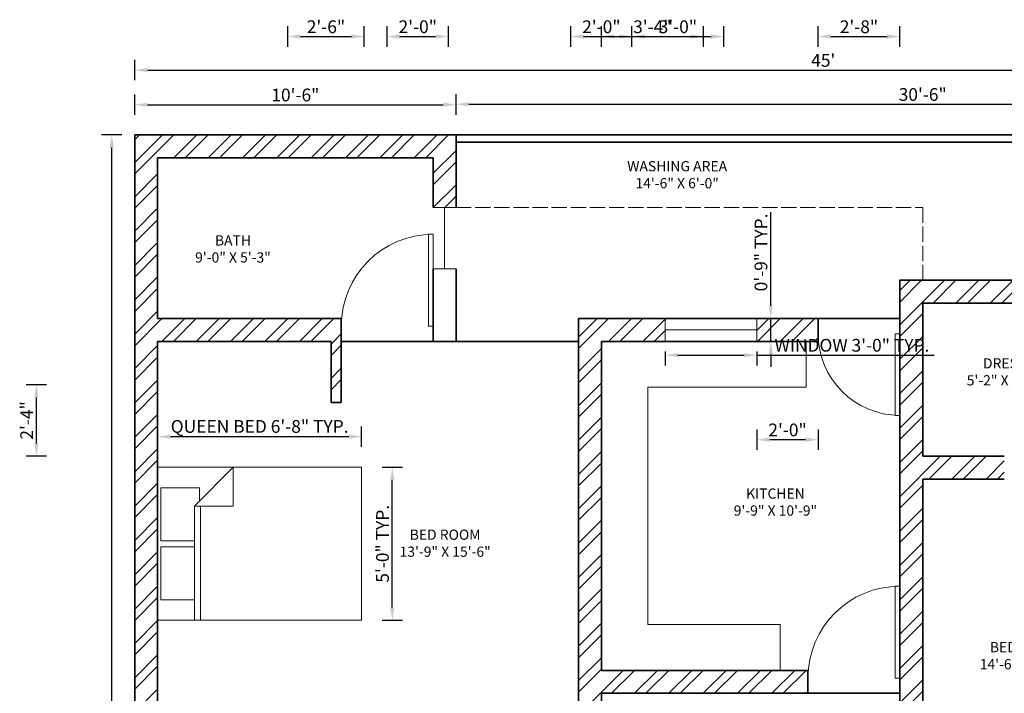
# Model space of a CAD drawing. Units: inches. Extents: x 468 to 1096, y 138 to 946.
# Tile 4 of 6: x 468 to 854, y 682 to 946. Entities that reach past the tile are written whole.
import ezdxf

# ---------------------------------------------------------------- set-up
doc = ezdxf.new("R2010")
doc.units = ezdxf.units.IN
doc.linetypes.add('ACAD_ISO02W100', pattern=[15, 12, -3])
for name, color, linetype, lineweight in [('A-ANNO-DIMS', 2, 'Continuous', 18), ('A-AREA-IDEN', 7, 'Continuous', 18), ('A-DOOR', 3, 'Continuous', 18), ('A-FLOR-CASE', 9, 'Continuous', 18), ('A-FURN', 8, 'Continuous', 18), ('A-GLAZ', 4, 'Continuous', 18), ('A-ROOF-OVHD', 7, 'ACAD_ISO02W100', 18), ('A-WALL', 7, 'Continuous', 35), ('A-WALL-PATT', 8, 'Continuous', 13), ('C-PROP', 7, 'Continuous', 35)]:
    doc.layers.add(name, color=color, linetype=linetype, lineweight=lineweight)
doc.styles.get("Standard").update_dxf_attribs({"font": 'arial.ttf'})
doc.dimstyles.new('ISO-25', dxfattribs={"dimtxt": 5, "dimasz": 5, "dimexe": 4, "dimexo": 4, "dimtad": 1, "dimdec": 1, "dimlunit": 3, "dimtxsty": 'Standard', "dimcen": 2.5, "dimadec": 0, "dimazin": 0, "dimtfac": 1, "dimtdec": 1, "dimtmove": 0, "dimatfit": 3, "dimfxl": 4, "dimfxlon": 1, "dimarcsym": 0})

# ---------------------------------------------------------------- blocks, each defined once
blk = doc.blocks.new('*U3')
for p, q in [((0, 0), (0, -6)), ((-36, 0), (-36, -6))]:
    blk.add_line(p, q)
blk.add_lwpolyline([(0, 0), (0, 36), (-1.75, 36), (-1.75, 0)], close=True)
blk.add_arc((0, 0), 36, 90, 180)
blk = doc.blocks.new('*U4')
for p, q in [((0, 0), (0, -6)), ((-32, 0), (-32, -6))]:
    blk.add_line(p, q)
blk.add_lwpolyline([(0, 0), (0, 32), (-1.75, 32), (-1.75, 0)], close=True)
blk.add_arc((0, 0), 32, 90, 180)
blk = doc.blocks.new('Bed - Queen')
for p, q in [((0, -80.00003), (0, 0)), ((0, 0), (59.99999, 0)), ((59.99999, 0), (59.99999, -80.00003)), ((7.99999, -1.2), (28.79998, -1.2)), ((7.99999, -14.4), (7.99999, -1.2)), ((28.79998, -1.2), (28.79998, -14.4)), ((31.19999, -1.2), (51.99999, -1.2)), ((31.19999, -14.4), (31.19999, -1.2)), ((51.99999, -1.2), (51.99999, -16.4)), ((0, -14.4), (44.8, -14.4)), ((59.99999, -29.6), (44.8, -14.4)), ((44.8, -14.4), (44.8, -29.6)), ((44.8, -16.8), (0, -16.8)), ((51.99999, -16.4), (46.79936, -16.4)), ((44.8, -29.6), (59.99999, -29.6)), ((59.99999, -80.00003), (0, -80.00003))]:
    blk.add_line(p, q)
blk = doc.blocks.new('*D15')
at = {"layer": 'A-ANNO-DIMS', "color": 0, "lineweight": -2, "transparency": 16777216}
for p, q in [((513.13, 908.95), (513.13, 916.95)), ((639.13, 908.95), (639.13, 916.95)), ((518.13, 912.95), (634.13, 912.95))]:
    blk.add_line(p, q, dxfattribs=at)
at = {"layer": 'A-ANNO-DIMS', "color": 0, "transparency": 16777216}
for points in [[(518.13, 913.79), (518.13, 912.12), (513.13, 912.95)], [(634.13, 913.79), (634.13, 912.12), (639.13, 912.95)]]:
    blk.add_solid(points, dxfattribs=at)
at = {"layer": 'Defpoints', "color": 0, "transparency": 16777216}
for p in [(639.13, 912.95), (513.13, 901.16), (639.13, 901.16)]:
    blk.add_point(p, dxfattribs=at)
at = {"layer": 'A-ANNO-DIMS', "color": 0, "transparency": 16777216, "insert": (576.13, 916.13), "char_height": 5, "attachment_point": 5}
blk.add_mtext('10\'-6"', dxfattribs=at)
blk = doc.blocks.new('*D16')
at = {"layer": 'A-ANNO-DIMS', "color": 0, "lineweight": -2, "transparency": 16777216}
for p, q in [((639.13, 909.15), (639.13, 917.15)), ((1005.13, 909.15), (1005.13, 917.15)), ((644.13, 913.15), (1000.13, 913.15))]:
    blk.add_line(p, q, dxfattribs=at)
at = {"layer": 'A-ANNO-DIMS', "color": 0, "transparency": 16777216}
for points in [[(644.13, 913.98), (644.13, 912.31), (639.13, 913.15)], [(1000.13, 913.98), (1000.13, 912.31), (1005.13, 913.15)]]:
    blk.add_solid(points, dxfattribs=at)
at = {"layer": 'Defpoints', "color": 0, "transparency": 16777216}
for p in [(1005.13, 913.15), (639.13, 901.16), (1005.13, 901.16)]:
    blk.add_point(p, dxfattribs=at)
at = {"layer": 'A-ANNO-DIMS', "color": 0, "transparency": 16777216, "insert": (822.13, 916.33), "char_height": 5, "attachment_point": 5}
blk.add_mtext('30\'-6"', dxfattribs=at)
blk = doc.blocks.new('*D18')
at = {"layer": 'A-ANNO-DIMS', "color": 0, "lineweight": -2, "transparency": 16777216}
for p, q in [((508.14, 901.16), (500.14, 901.16)), ((504.14, 186.16), (504.14, 896.16)), ((508.14, 181.16), (500.14, 181.16))]:
    blk.add_line(p, q, dxfattribs=at)
at = {"layer": 'A-ANNO-DIMS', "color": 0, "transparency": 16777216}
for points in [[(503.3, 896.16), (504.97, 896.16), (504.14, 901.16)], [(503.3, 186.16), (504.97, 186.16), (504.14, 181.16)]]:
    blk.add_solid(points, dxfattribs=at)
at = {"layer": 'Defpoints', "color": 0, "transparency": 16777216}
for p in [(504.14, 901.16), (513.13, 901.16), (513.13, 181.16)]:
    blk.add_point(p, dxfattribs=at)
at = {"layer": 'A-ANNO-DIMS', "color": 0, "transparency": 16777216, "insert": (500.96, 541.16), "char_height": 5, "attachment_point": 5, "rotation": 90}
blk.add_mtext("60'", dxfattribs=at)
blk = doc.blocks.new('*D30')
at = {"layer": 'A-ANNO-DIMS', "color": 0, "lineweight": -2, "transparency": 16777216}
for p, q in [((513.13, 922.53), (513.13, 930.53)), ((1053.13, 922.53), (1053.13, 930.53)), ((518.13, 926.53), (1048.13, 926.53))]:
    blk.add_line(p, q, dxfattribs=at)
at = {"layer": 'A-ANNO-DIMS', "color": 0, "transparency": 16777216}
for points in [[(518.13, 927.37), (518.13, 925.7), (513.13, 926.53)], [(1048.13, 927.37), (1048.13, 925.7), (1053.13, 926.53)]]:
    blk.add_solid(points, dxfattribs=at)
at = {"layer": 'Defpoints', "color": 0, "transparency": 16777216}
for p in [(1053.13, 926.53), (513.13, 901.16), (1053.13, 901.16)]:
    blk.add_point(p, dxfattribs=at)
at = {"layer": 'A-ANNO-DIMS', "color": 0, "transparency": 16777216, "insert": (783.13, 929.7), "char_height": 5, "attachment_point": 5}
blk.add_mtext("45'", dxfattribs=at)
blk = doc.blocks.new('WIN-24-W9')
for p, q in [((0, 24), (9, 24)), ((4.5, 24), (4.5, 0)), ((0, 0), (9, 0))]:
    blk.add_line(p, q)
blk = doc.blocks.new('WIN-36-W9')
for p, q in [((0, 9), (0, 0)), ((36, 9), (36, 0)), ((0, 4.5), (36, 4.5))]:
    blk.add_line(p, q)
blk = doc.blocks.new('*D35')
at = {"layer": 'A-ANNO-DIMS', "color": 0, "lineweight": -2, "transparency": 16777216}
for p, q in [((522.13, 778.79), (522.13, 786.79)), ((602.13, 778.79), (602.13, 786.79)), ((597.13, 782.79), (527.13, 782.79))]:
    blk.add_line(p, q, dxfattribs=at)
at = {"layer": 'A-ANNO-DIMS', "color": 0, "transparency": 16777216}
for points in [[(527.13, 783.63), (527.13, 781.96), (522.13, 782.79)], [(597.13, 783.63), (597.13, 781.96), (602.13, 782.79)]]:
    blk.add_solid(points, dxfattribs=at)
at = {"layer": 'Defpoints', "color": 0, "transparency": 16777216}
for p in [(522.13, 782.79), (522.13, 770.79), (602.13, 770.79)]:
    blk.add_point(p, dxfattribs=at)
at = {"layer": 'A-ANNO-DIMS', "color": 0, "transparency": 16777216, "insert": (562.13, 786.16), "char_height": 5, "attachment_point": 5}
blk.add_mtext('QUEEN BED 6\'-8" TYP.', dxfattribs=at)
blk = doc.blocks.new('*D36')
at = {"layer": 'A-ANNO-DIMS', "color": 0, "lineweight": -2, "transparency": 16777216}
for p, q in [((610.13, 770.79), (618.13, 770.79)), ((614.13, 715.79), (614.13, 765.79)), ((610.13, 710.79), (618.13, 710.79))]:
    blk.add_line(p, q, dxfattribs=at)
at = {"layer": 'A-ANNO-DIMS', "color": 0, "transparency": 16777216}
for points in [[(613.3, 765.79), (614.96, 765.79), (614.13, 770.79)], [(613.3, 715.79), (614.96, 715.79), (614.13, 710.79)]]:
    blk.add_solid(points, dxfattribs=at)
at = {"layer": 'Defpoints', "color": 0, "transparency": 16777216}
for p in [(602.13, 770.79), (614.13, 770.79), (602.13, 710.79)]:
    blk.add_point(p, dxfattribs=at)
at = {"layer": 'A-ANNO-DIMS', "color": 0, "transparency": 16777216, "insert": (610.95, 740.79), "char_height": 5, "attachment_point": 5, "rotation": 90}
blk.add_mtext('5\'-0" TYP.', dxfattribs=at)
blk = doc.blocks.new('*D41')
at = {"layer": 'A-ANNO-DIMS', "color": 0, "lineweight": -2, "transparency": 16777216}
for p, q in [((721.13, 816.16), (721.13, 810.76)), ((726.13, 814.76), (752.13, 814.76)), ((757.13, 816.16), (757.13, 810.76)), ((757.13, 814.76), (826.65, 814.76))]:
    blk.add_line(p, q, dxfattribs=at)
at = {"layer": 'A-ANNO-DIMS', "color": 0, "transparency": 16777216}
for points in [[(726.13, 815.59), (726.13, 813.93), (721.13, 814.76)], [(752.13, 815.59), (752.13, 813.93), (757.13, 814.76)]]:
    blk.add_solid(points, dxfattribs=at)
at = {"layer": 'Defpoints', "color": 0, "transparency": 16777216}
for p in [(721.13, 820.16), (757.13, 820.16), (757.13, 814.76)]:
    blk.add_point(p, dxfattribs=at)
at = {"layer": 'A-ANNO-DIMS', "color": 0, "transparency": 16777216, "insert": (794.39, 817.98), "char_height": 5, "attachment_point": 5}
blk.add_mtext('WINDOW 3\'-0" TYP.', dxfattribs=at)
blk = doc.blocks.new('*D42')
at = {"layer": 'A-ANNO-DIMS', "color": 0, "lineweight": -2, "transparency": 16777216}
for p, q in [((762.53, 834.16), (762.53, 870.89)), ((761.13, 829.16), (766.53, 829.16)), ((762.53, 820.16), (762.53, 829.16)), ((761.13, 820.16), (766.53, 820.16)), ((762.53, 815.16), (762.53, 810.16))]:
    blk.add_line(p, q, dxfattribs=at)
at = {"layer": 'A-ANNO-DIMS', "color": 0, "transparency": 16777216}
for points in [[(761.7, 834.16), (763.36, 834.16), (762.53, 829.16)], [(761.7, 815.16), (763.36, 815.16), (762.53, 820.16)]]:
    blk.add_solid(points, dxfattribs=at)
at = {"layer": 'Defpoints', "color": 0, "transparency": 16777216}
for p in [(757.13, 829.16), (762.53, 829.16), (757.13, 820.16)]:
    blk.add_point(p, dxfattribs=at)
at = {"layer": 'A-ANNO-DIMS', "color": 0, "transparency": 16777216, "insert": (759.35, 855.03), "char_height": 5, "attachment_point": 5, "rotation": 90}
blk.add_mtext('0\'-9" TYP.', dxfattribs=at)
blk = doc.blocks.new('*D61')
at = {"layer": 'A-ANNO-DIMS', "color": 0, "lineweight": -2, "transparency": 16777216}
for p, q in [((594.13, 146.61), (594.13, 138.61)), ((630.13, 146.61), (630.13, 138.61)), ((599.13, 142.61), (625.13, 142.61))]:
    blk.add_line(p, q, dxfattribs=at)
at = {"layer": 'A-ANNO-DIMS', "color": 0, "transparency": 16777216}
for points in [[(599.13, 143.44), (599.13, 141.78), (594.13, 142.61)], [(625.13, 143.44), (625.13, 141.78), (630.13, 142.61)]]:
    blk.add_solid(points, dxfattribs=at)
at = {"layer": 'Defpoints', "color": 0, "transparency": 16777216}
for p in [(594.13, 829.16), (630.13, 826.16), (630.13, 142.61)]:
    blk.add_point(p, dxfattribs=at)
at = {"layer": 'A-ANNO-DIMS', "color": 0, "transparency": 16777216, "insert": (612.13, 145.79), "char_height": 5, "attachment_point": 5}
blk.add_mtext('3\'-0"', dxfattribs=at)
blk = doc.blocks.new('*D62')
at = {"layer": 'A-ANNO-DIMS', "color": 0, "lineweight": -2, "transparency": 16777216}
for p, q in [((781.13, 935.71), (781.13, 943.71)), ((813.13, 935.71), (813.13, 943.71)), ((786.13, 939.71), (808.13, 939.71))]:
    blk.add_line(p, q, dxfattribs=at)
at = {"layer": 'A-ANNO-DIMS', "color": 0, "transparency": 16777216}
for points in [[(786.13, 940.54), (786.13, 938.88), (781.13, 939.71)], [(808.13, 940.54), (808.13, 938.88), (813.13, 939.71)]]:
    blk.add_solid(points, dxfattribs=at)
at = {"layer": 'Defpoints', "color": 0, "transparency": 16777216}
for p in [(813.13, 939.71), (781.13, 829.16), (813.13, 829.16)]:
    blk.add_point(p, dxfattribs=at)
at = {"layer": 'A-ANNO-DIMS', "color": 0, "transparency": 16777216, "insert": (797.13, 942.89), "char_height": 5, "attachment_point": 5}
blk.add_mtext('2\'-8"', dxfattribs=at)
blk = doc.blocks.new('*D65')
at = {"layer": 'A-ANNO-DIMS', "color": 0, "lineweight": -2, "transparency": 16777216}
for p, q in [((478.58, 803.16), (470.58, 803.16)), ((474.58, 780.16), (474.58, 798.16)), ((478.58, 775.16), (470.58, 775.16))]:
    blk.add_line(p, q, dxfattribs=at)
at = {"layer": 'A-ANNO-DIMS', "color": 0, "transparency": 16777216}
for points in [[(473.75, 798.16), (475.41, 798.16), (474.58, 803.16)], [(473.75, 780.16), (475.41, 780.16), (474.58, 775.16)]]:
    blk.add_solid(points, dxfattribs=at)
at = {"layer": 'Defpoints', "color": 0, "transparency": 16777216}
for p in [(474.58, 803.16), (884.13, 803.16), (884.13, 775.16)]:
    blk.add_point(p, dxfattribs=at)
at = {"layer": 'A-ANNO-DIMS', "color": 0, "transparency": 16777216, "insert": (471.44, 789.16), "char_height": 5, "attachment_point": 5, "rotation": 90}
blk.add_mtext('2\'-4"', dxfattribs=at)
blk = doc.blocks.new('*D66')
at = {"layer": 'A-ANNO-DIMS', "color": 0, "lineweight": -2, "transparency": 16777216}
for p, q in [((696.13, 146.61), (696.13, 138.61)), ((714.39, 146.61), (714.39, 138.61)), ((701.13, 142.61), (709.39, 142.61)), ((714.39, 142.61), (745.11, 142.61))]:
    blk.add_line(p, q, dxfattribs=at)
at = {"layer": 'A-ANNO-DIMS', "color": 0, "transparency": 16777216}
for points in [[(701.13, 143.44), (701.13, 141.78), (696.13, 142.61)], [(709.39, 143.44), (709.39, 141.78), (714.39, 142.61)]]:
    blk.add_solid(points, dxfattribs=at)
at = {"layer": 'Defpoints', "color": 0, "transparency": 16777216}
for p in [(696.13, 820.16), (714.39, 802.16), (714.39, 142.61)]:
    blk.add_point(p, dxfattribs=at)
at = {"layer": 'A-ANNO-DIMS', "color": 0, "transparency": 16777216, "insert": (732.25, 145.82), "char_height": 5, "attachment_point": 5}
blk.add_mtext('1\'-6 1/2"', dxfattribs=at)
blk = doc.blocks.new('*D75')
at = {"layer": 'A-ANNO-DIMS', "color": 0, "lineweight": -2, "transparency": 16777216}
for p, q in [((696.13, 935.71), (696.13, 943.71)), ((736.13, 935.71), (736.13, 943.71)), ((701.13, 939.71), (731.13, 939.71))]:
    blk.add_line(p, q, dxfattribs=at)
at = {"layer": 'A-ANNO-DIMS', "color": 0, "transparency": 16777216}
for points in [[(701.13, 940.54), (701.13, 938.88), (696.13, 939.71)], [(731.13, 940.54), (731.13, 938.88), (736.13, 939.71)]]:
    blk.add_solid(points, dxfattribs=at)
at = {"layer": 'Defpoints', "color": 0, "transparency": 16777216}
for p in [(736.13, 939.71), (696.13, 412.16), (736.13, 412.16)]:
    blk.add_point(p, dxfattribs=at)
at = {"layer": 'A-ANNO-DIMS', "color": 0, "transparency": 16777216, "insert": (716.13, 942.89), "char_height": 5, "attachment_point": 5}
blk.add_mtext('3\'-4"', dxfattribs=at)
blk = doc.blocks.new('*D78')
at = {"layer": 'A-ANNO-DIMS', "color": 0, "lineweight": -2, "transparency": 16777216}
for p, q in [((573.13, 935.71), (573.13, 943.71)), ((603.13, 935.71), (603.13, 943.71)), ((578.13, 939.71), (598.13, 939.71))]:
    blk.add_line(p, q, dxfattribs=at)
at = {"layer": 'A-ANNO-DIMS', "color": 0, "transparency": 16777216}
for points in [[(578.13, 940.54), (578.13, 938.88), (573.13, 939.71)], [(598.13, 940.54), (598.13, 938.88), (603.13, 939.71)]]:
    blk.add_solid(points, dxfattribs=at)
at = {"layer": 'Defpoints', "color": 0, "transparency": 16777216}
for p in [(603.13, 939.71), (573.13, 250.16), (603.13, 250.16)]:
    blk.add_point(p, dxfattribs=at)
at = {"layer": 'A-ANNO-DIMS', "color": 0, "transparency": 16777216, "insert": (588.13, 942.89), "char_height": 5, "attachment_point": 5}
blk.add_mtext('2\'-6"', dxfattribs=at)
blk = doc.blocks.new('*D79')
at = {"layer": 'A-ANNO-DIMS', "color": 0, "lineweight": -2, "transparency": 16777216}
for p, q in [((612.13, 935.71), (612.13, 943.71)), ((636.13, 935.71), (636.13, 943.71)), ((617.13, 939.71), (631.13, 939.71))]:
    blk.add_line(p, q, dxfattribs=at)
at = {"layer": 'A-ANNO-DIMS', "color": 0, "transparency": 16777216}
for points in [[(617.13, 940.54), (617.13, 938.88), (612.13, 939.71)], [(631.13, 940.54), (631.13, 938.88), (636.13, 939.71)]]:
    blk.add_solid(points, dxfattribs=at)
at = {"layer": 'Defpoints', "color": 0, "transparency": 16777216}
for p in [(636.13, 939.71), (612.13, 241.16), (636.13, 241.16)]:
    blk.add_point(p, dxfattribs=at)
at = {"layer": 'A-ANNO-DIMS', "color": 0, "transparency": 16777216, "insert": (624.13, 942.89), "char_height": 5, "attachment_point": 5}
blk.add_mtext('2\'-0"', dxfattribs=at)
blk = doc.blocks.new('*D80')
at = {"layer": 'A-ANNO-DIMS', "color": 0, "lineweight": -2, "transparency": 16777216}
for p, q in [((684.13, 935.71), (684.13, 943.71)), ((708.13, 935.71), (708.13, 943.71)), ((689.13, 939.71), (703.13, 939.71))]:
    blk.add_line(p, q, dxfattribs=at)
at = {"layer": 'A-ANNO-DIMS', "color": 0, "transparency": 16777216}
for points in [[(689.13, 940.54), (689.13, 938.88), (684.13, 939.71)], [(703.13, 940.54), (703.13, 938.88), (708.13, 939.71)]]:
    blk.add_solid(points, dxfattribs=at)
at = {"layer": 'Defpoints', "color": 0, "transparency": 16777216}
for p in [(708.13, 939.71), (684.13, 250.16), (708.13, 250.16)]:
    blk.add_point(p, dxfattribs=at)
at = {"layer": 'A-ANNO-DIMS', "color": 0, "transparency": 16777216, "insert": (696.13, 942.89), "char_height": 5, "attachment_point": 5}
blk.add_mtext('2\'-0"', dxfattribs=at)
blk = doc.blocks.new('*D81')
at = {"layer": 'A-ANNO-DIMS', "color": 0, "lineweight": -2, "transparency": 16777216}
for p, q in [((708.13, 935.71), (708.13, 943.71)), ((744.13, 935.71), (744.13, 943.71)), ((713.13, 939.71), (739.13, 939.71))]:
    blk.add_line(p, q, dxfattribs=at)
at = {"layer": 'A-ANNO-DIMS', "color": 0, "transparency": 16777216}
for points in [[(713.13, 940.54), (713.13, 938.88), (708.13, 939.71)], [(739.13, 940.54), (739.13, 938.88), (744.13, 939.71)]]:
    blk.add_solid(points, dxfattribs=at)
at = {"layer": 'Defpoints', "color": 0, "transparency": 16777216}
for p in [(744.13, 939.71), (708.13, 250.16), (744.13, 250.16)]:
    blk.add_point(p, dxfattribs=at)
at = {"layer": 'A-ANNO-DIMS', "color": 0, "transparency": 16777216, "insert": (726.13, 942.89), "char_height": 5, "attachment_point": 5}
blk.add_mtext('3\'-0"', dxfattribs=at)
blk = doc.blocks.new('*D84')
at = {"layer": 'A-ANNO-DIMS', "color": 0, "lineweight": -2, "transparency": 16777216}
for p, q in [((757.13, 785.61), (757.13, 777.61)), ((781.13, 785.61), (781.13, 777.61)), ((776.13, 781.61), (762.13, 781.61))]:
    blk.add_line(p, q, dxfattribs=at)
at = {"layer": 'A-ANNO-DIMS', "color": 0, "transparency": 16777216}
for points in [[(762.13, 782.44), (762.13, 780.78), (757.13, 781.61)], [(776.13, 782.44), (776.13, 780.78), (781.13, 781.61)]]:
    blk.add_solid(points, dxfattribs=at)
at = {"layer": 'Defpoints', "color": 0, "transparency": 16777216}
for p in [(757.13, 820.16), (781.13, 820.16), (757.13, 781.61)]:
    blk.add_point(p, dxfattribs=at)
at = {"layer": 'A-ANNO-DIMS', "color": 0, "transparency": 16777216, "insert": (769.13, 784.79), "char_height": 5, "attachment_point": 5}
blk.add_mtext('2\'-0"', dxfattribs=at)

msp = doc.modelspace()

# ---------------------------------------------------------------- hatches: boundary and pattern name
at = {"layer": 'A-WALL-PATT'}
h = msp.add_hatch(dxfattribs=at)
h.set_pattern_fill('ANSI32', color=256)
h.paths.add_polyline_path([(639.13, 901.16), (513.13, 901.16), (513.13, 181.16), (612.13, 181.16), (612.13, 202.16), (603.13, 202.16), (603.13, 190.16), (522.13, 190.16), (522.13, 241.16), (573.13, 241.16), (573.13, 250.16), (522.13, 250.16), (522.13, 403.16), (696.13, 403.16), (696.13, 418.16), (687.13, 418.16), (687.13, 412.16), (615.37, 412.16), (615.37, 436.16), (611.37, 436.16), (611.37, 412.16), (522.13, 412.16), (522.13, 436.16), (522.13, 565.16), (528.13, 565.16), (528.13, 571.16), (522.13, 571.16), (522.13, 625.16), (531.13, 625.16), (531.13, 634.16), (522.13, 634.16), (522.13, 820.16), (590.13, 820.16), (590.13, 796.16), (594.13, 796.16), (594.13, 820.16), (594.13, 826.16), (594.13, 829.16), (522.13, 829.16), (522.13, 892.16), (630.13, 892.16), (630.13, 872.66), (639.13, 872.66)])
h = msp.add_hatch(dxfattribs=at)
h.set_pattern_fill('ANSI32', color=256)
h.paths.add_polyline_path([(696.13, 634.16), (687.13, 634.16), (650.13, 634.16), (567.13, 634.16), (567.13, 625.16), (573.13, 625.16), (573.13, 610.16), (579.13, 610.16), (579.13, 625.16), (687.13, 625.16), (687.13, 454.16), (696.13, 454.16), (696.13, 598.16), (813.13, 598.16), (813.13, 607.16), (696.13, 607.16)])
h.paths.add_polyline_path([(777.13, 688.16), (777.13, 691.16), (696.13, 691.16), (696.13, 820.16), (721.13, 820.16), (721.13, 829.16), (687.13, 829.16), (687.13, 820.16), (687.13, 674.16), (696.13, 674.16), (696.13, 682.16), (777.13, 682.16)])
h.paths.add_polyline_path([(854.13, 775.16), (822.13, 775.16), (822.13, 835.16), (884.13, 835.16), (884.13, 803.19), (888.13, 803.19), (888.13, 835.16), (987.13, 835.16), (987.13, 817.16), (996.13, 817.16), (996.13, 844.16), (987.13, 844.16), (813.13, 844.16), (813.13, 829.16), (813.13, 823.16), (813.13, 791.16), (813.13, 691.16), (813.13, 688.16), (813.13, 682.16), (813.13, 643.16), (819.13, 643.16), (822.13, 643.16), (822.13, 691.16), (822.13, 766.16), (854.13, 766.16)])
h.paths.add_polyline_path([(996.13, 775.16), (996.13, 784.16), (996.13, 793.16), (987.13, 793.16), (987.13, 775.16), (884.13, 775.16), (884.13, 766.16), (987.13, 766.16), (987.13, 718.16), (996.13, 718.16)], flags=17)
h.paths.add_polyline_path([(781.13, 829.16), (757.13, 829.16), (757.13, 820.16), (781.13, 820.16)])

# ---------------------------------------------------------------- linework, layer by layer
at = {"layer": 'A-FLOR-CASE'}
for p, q in [((776.39, 820.16), (776.39, 802.16)), ((776.39, 802.16), (714.39, 802.16)), ((714.39, 802.16), (714.39, 718.16)), ((714.39, 718.16), (714.39, 715.16)), ((714.39, 715.16), (714.39, 709.16)), ((714.39, 709.16), (766.19, 709.16)), ((766.19, 709.16), (766.19, 691.16))]:
    msp.add_line(p, q, dxfattribs=at)
at = {"layer": 'A-ROOF-OVHD', "ltscale": 0.5}
for p, q in [((639.13, 872.66), (822.13, 872.66)), ((822.13, 872.66), (822.13, 844.16))]:
    msp.add_line(p, q, dxfattribs=at)
at = {"layer": 'A-WALL'}
for p, q in [((639.13, 901.16), (639.13, 872.66)), ((522.13, 892.16), (522.13, 829.16)), ((630.13, 892.16), (522.13, 892.16)), ((630.13, 892.16), (630.13, 872.66)), ((630.13, 848.66), (630.13, 820.16)), ((639.13, 848.66), (639.13, 820.16)), ((822.13, 775.16), (822.13, 835.16)), ((822.13, 835.16), (884.13, 835.16)), ((594.13, 829.16), (522.13, 829.16)), ((594.13, 829.16), (594.13, 820.16)), ((687.13, 820.16), (687.13, 829.16)), ((687.13, 829.16), (813.13, 829.16)), ((781.13, 829.16), (781.13, 820.16)), ((813.13, 820.16), (813.13, 829.16)), ((522.13, 820.16), (522.13, 634.16)), ((590.13, 820.16), (522.13, 820.16)), ((590.13, 796.16), (590.13, 820.16)), ((639.13, 820.16), (594.13, 820.16)), ((594.13, 820.16), (594.13, 796.16)), ((639.13, 820.16), (687.13, 820.16)), ((687.13, 820.16), (687.13, 674.16)), ((696.13, 820.16), (696.13, 691.16)), ((696.13, 820.16), (781.13, 820.16)), ((594.13, 796.16), (590.13, 796.16)), ((822.13, 775.16), (854.13, 775.16)), ((822.13, 691.16), (822.13, 766.16)), ((822.13, 766.16), (854.13, 766.16)), ((777.13, 691.16), (696.13, 691.16)), ((777.13, 691.16), (777.13, 682.16)), ((813.13, 691.16), (813.13, 682.16)), ((822.13, 643.16), (822.13, 691.16)), ((813.13, 682.16), (696.13, 682.16)), ((696.13, 682.16), (696.13, 674.16))]:
    msp.add_line(p, q, dxfattribs=at)
for points in [[(813.13, 829.16), (813.13, 844.16), (987.13, 844.16), (996.13, 844.16), (996.13, 784.16), (996.13, 775.16), (996.13, 607.16), (996.13, 598.16)], [(813.13, 691.16), (813.13, 820.16)], [(813.13, 643.16), (813.13, 682.16)]]:
    msp.add_lwpolyline(points, dxfattribs=at)
at = {"layer": 'C-PROP'}
for p, q in [((1053.13, 901.16), (513.13, 901.16)), ((513.13, 901.16), (513.13, 181.16)), ((1050.72, 898.26), (639.13, 898.26))]:
    msp.add_line(p, q, dxfattribs=at)

# ---------------------------------------------------------------- block references
at = {"layer": 'A-DOOR'}
for p in [(630.13, 826.16), (813.13, 688.16)]:
    msp.add_blockref('*U3', p, dxfattribs=at)
at = {"layer": 'A-DOOR', "xscale": -1, "rotation": 180}
msp.add_blockref('*U4', (813.13, 823.16), dxfattribs=at)
at = {"layer": 'A-FURN', "rotation": 90}
msp.add_blockref('Bed - Queen', (522.13, 710.79), dxfattribs=at)
at = {"layer": 'A-GLAZ'}
for name, p in [('WIN-24-W9', (630.13, 848.66)), ('WIN-36-W9', (721.13, 820.16))]:
    msp.add_blockref(name, p, dxfattribs=at)

# ---------------------------------------------------------------- texts
at = {"layer": 'A-AREA-IDEN', "char_height": 4, "attachment_point": 1}
for s, width, insert in [('\\pxqc;WASHING AREA\\P14\'-6" X 6\'-0"', 44.9099, (703.39, 890.85)), ('\\pxqc;BATH\\P9\'-0" X 5\'-3"', 36.2598, (533.54, 861.74)), ('\\pxqc;DRESS\\P5\'-2" X 5\'-0"', 36.2598, (836.11, 813.55)), ('\\pxqc;KITCHEN\\P9\'-9" X 10\'-9"', 36.2598, (746.25, 762.48)), ('\\pxqc;BED ROOM\\P13\'-9" X 15\'-6"', 36.2598, (616.74, 746.36)), ('\\pxqc;BED ROOM\\P14\'-6" X 14\'-0"', 36.2598, (844.23, 702.25))]:
    msp.add_mtext_dynamic_manual_height_columns(s, width=width, gutter_width=12.5, heights=[0], dxfattribs=dict(at, insert=insert))

# ---------------------------------------------------------------- dimensions: what is measured, and where the dimension line sits
at = {"layer": 'A-ANNO-DIMS'}
for base, p1, p2, override, picture, middle in [((603.13, 939.71), (573.13, 250.16), (603.13, 250.16), {"dimdec": 1, "dimlfac": 1, "dimrnd": 0, "dimzin": 1, "dimdsep": 46, "dimlunit": 4, "dimfrac": 2}, '*D78', (588.13, 942.89)), ((636.13, 939.71), (612.13, 241.16), (636.13, 241.16), {"dimdec": 1, "dimlfac": 1, "dimrnd": 0, "dimzin": 1, "dimdsep": 46, "dimlunit": 4, "dimfrac": 2}, '*D79', (624.13, 942.89)), ((708.13, 939.71), (684.13, 250.16), (708.13, 250.16), {"dimdec": 1, "dimlfac": 1, "dimrnd": 0, "dimzin": 1, "dimdsep": 46, "dimlunit": 4, "dimfrac": 2}, '*D80', (696.13, 942.89)), ((736.13, 939.71), (696.13, 412.16), (736.13, 412.16), {"dimdec": 1, "dimlfac": 1, "dimrnd": 0, "dimzin": 1, "dimdsep": 46, "dimlunit": 4, "dimfrac": 2}, '*D75', (716.13, 942.89)), ((744.13, 939.71), (708.13, 250.16), (744.13, 250.16), {"dimdec": 1, "dimlfac": 1, "dimrnd": 0, "dimzin": 1, "dimdsep": 46, "dimlunit": 4, "dimfrac": 2}, '*D81', (726.13, 942.89)), ((813.13, 939.71), (781.13, 829.16), (813.13, 829.16), {"dimdec": 1, "dimlfac": 1, "dimrnd": 0, "dimzin": 1, "dimdsep": 46, "dimlunit": 4, "dimfrac": 2}, '*D62', (797.13, 942.89)), ((1053.13, 926.53), (513.13, 901.16), (1053.13, 901.16), {"dimclrd": 0, "dimclre": 0, "dimclrt": 0}, '*D30', (783.13, 929.7)), ((639.13, 912.95), (513.13, 901.16), (639.13, 901.16), {"dimclrd": 0, "dimclre": 0, "dimclrt": 0}, '*D15', (576.13, 916.13)), ((1005.13, 913.15), (639.13, 901.16), (1005.13, 901.16), {"dimclrd": 0, "dimclre": 0, "dimclrt": 0}, '*D16', (822.13, 916.33)), ((630.13, 142.61), (594.13, 829.16), (630.13, 826.16), {"dimdec": 1, "dimlfac": 1, "dimrnd": 0, "dimzin": 1, "dimdsep": 46, "dimlunit": 4, "dimfrac": 2}, '*D61', (612.13, 145.79)), ((714.39, 142.61), (696.13, 820.16), (714.39, 802.16), {"dimdec": 1, "dimlfac": 1, "dimrnd": 0, "dimzin": 1, "dimdsep": 46, "dimlunit": 4, "dimfrac": 2}, '*D66', (732.25, 145.82))]:
    dim = msp.add_linear_dim(base=base, p1=p1, p2=p2, dimstyle='ISO-25', override=override, dxfattribs=at)
    dim.commit()
    dim.dimension.update_dxf_attribs({"geometry": picture, "text_midpoint": middle})
for base, p1, p2, angle, override, picture, middle in [((504.14, 901.16), (513.13, 181.16), (513.13, 901.16), 90, {"dimclrd": 0, "dimclre": 0, "dimclrt": 0}, '*D18', (500.96, 541.16)), ((757.13, 781.61), (781.13, 820.16), (757.13, 820.16), 180, {"dimdec": 1, "dimlfac": 1, "dimrnd": 0, "dimzin": 1, "dimdsep": 46, "dimlunit": 4, "dimfrac": 2}, '*D84', (769.13, 784.79)), ((474.58, 803.16), (884.13, 775.16), (884.13, 803.16), 90, {"dimdec": 1, "dimlfac": 1, "dimrnd": 0, "dimzin": 1, "dimdsep": 46, "dimlunit": 4, "dimfrac": 2}, '*D65', (471.44, 789.16))]:
    dim = msp.add_linear_dim(base=base, p1=p1, p2=p2, angle=angle, dimstyle='ISO-25', override=override, dxfattribs=at)
    dim.commit()
    dim.dimension.update_dxf_attribs({"geometry": picture, "text_midpoint": middle})
for base, p1, p2, angle, text, picture, middle in [((762.53, 829.16), (757.13, 820.16), (757.13, 829.16), 90, '<> TYP.', '*D42', (759.35, 855.03)), ((522.13, 782.79), (602.13, 770.79), (522.13, 770.79), 180, 'QUEEN BED <> TYP.', '*D35', (562.13, 786.16)), ((614.13, 770.79), (602.13, 710.79), (602.13, 770.79), 90, '<> TYP.', '*D36', (610.95, 740.79))]:
    dim = msp.add_linear_dim(base=base, p1=p1, p2=p2, angle=angle, text=text, dimstyle='ISO-25', override={"dimdec": 1, "dimlfac": 1, "dimrnd": 0, "dimzin": 1, "dimdsep": 46, "dimlunit": 4, "dimfrac": 2}, dxfattribs=at)
    dim.commit()
    dim.dimension.update_dxf_attribs({"geometry": picture, "text_midpoint": middle})
dim = msp.add_linear_dim(base=(757.13, 814.76), p1=(721.13, 820.16), p2=(757.13, 820.16), text='WINDOW <> TYP.', dimstyle='ISO-25', override={"dimdec": 1, "dimlfac": 1, "dimrnd": 0, "dimzin": 1, "dimdsep": 46, "dimlunit": 4, "dimfrac": 2}, dxfattribs=at)
dim.commit()
dim.dimension.update_dxf_attribs({"geometry": '*D41', "text_midpoint": (794.39, 817.98)})

doc.saveas('drawing.dxf')
